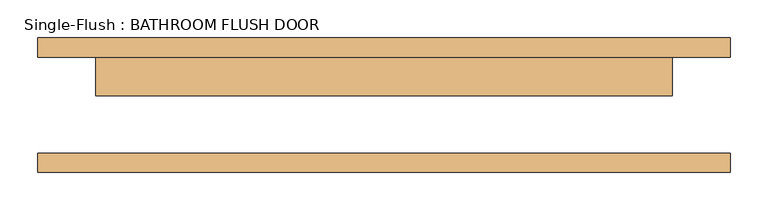
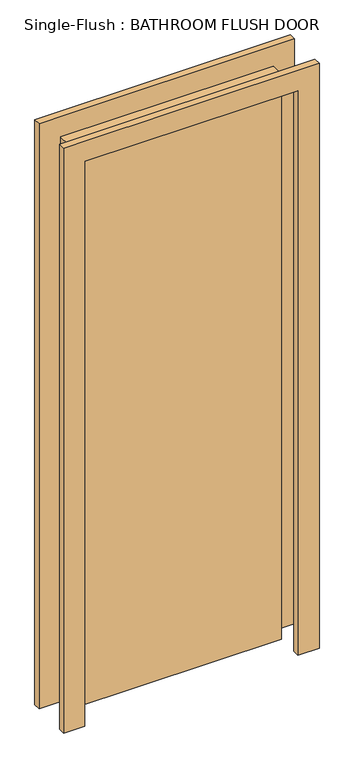
"""IFC4 building model written with IfcOpenShell, lengths in millimetres: door geometry, Single-Flush : BATHROOM FLUSH DOOR."""

from ifc_helpers import new_model, si_unit, frame, origin, origin_with_axes, place, context, project, spatial, polyline, outline, extrude, source, transform, mapped, element, save


def single_flush_bathroom_flush_door_4d6c7550(model_context):
    return source(origin(), model_context, "Body", "SweptSolid", [
        extrude(outline(polyline([(2209.8, -457.2), (0.0, -457.2), (0.0, -381.0), (2133.6, -381.0), (2133.6, 381.0), (0.0, 381.0), (0.0, 457.2), (2209.8, 457.2), (2209.8, -457.2)])), frame((0.0, 63.5, 0.0), z_axis=(0.0, 1.0, 0.0), x_axis=(0.0, 0.0, 1.0)), (0.0, 0.0, 1.0), 25.4),
        extrude(outline(polyline([(2209.8, 457.2), (2209.8, -457.2), (0.0, -457.2), (0.0, -381.0), (2133.6, -381.0), (2133.6, 381.0), (0.0, 381.0), (0.0, 457.2), (2209.8, 457.2)])), frame((0.0, -88.9, 0.0), z_axis=(0.0, 1.0, 0.0), x_axis=(0.0, 0.0, 1.0)), (0.0, 0.0, 1.0), 25.4),
        extrude(outline(polyline([(381.0, 12.7), (-381.0, 12.7), (-381.0, 63.5), (381.0, 63.5), (381.0, 12.7)])), origin_with_axes(), (0.0, 0.0, 1.0), 2133.6),
    ])


if __name__ == "__main__":
    model = new_model("IFC4")
    model_context = context("Model", 3, world=origin())
    ifc_project = project(units=[si_unit("LENGTHUNIT", "METRE", prefix="MILLI")], contexts=[model_context])
    site = spatial("IfcSite", under=ifc_project)
    building = spatial("IfcBuilding", under=site)
    placement = place(None, origin())
    single_flush_bathroom_flush_door_shape = single_flush_bathroom_flush_door_4d6c7550(model_context)
    element("IfcDoor", 1, ObjectType="Single-Flush : BATHROOM FLUSH DOOR", at=placement, inside=building, context=model_context, shape_type="MappedRepresentation", body=[
        mapped(single_flush_bathroom_flush_door_shape, transform((0.0, 0.0, 0.0), x_axis=(1.0, 0.0, 0.0), y_axis=(0.0, 1.0, 0.0), z_axis=(0.0, 0.0, 1.0))),
    ])
    save(model, "model.ifc")

# Revit data of these elements
# Type "Single-Flush : BATHROOM FLUSH DOOR"
#   Type Mark = "9"
#   Construction Type Id = "MDOOR"
#   Assembly Code = "C1020"
#   Analytic Construction = "Metal"
#   Thickness = 0' - 2"
#   Heat Transfer Coefficient (U) = 0.651978 BTU/(h·ft²·°F)
#   Height = 7' - 0"
#   Trim Projection Ext = 0' - 1"
#   Trim Projection Int = 0' - 1"
#   Trim Width = 0' - 3"
#   Width = 2' - 6"
#   Define Thermal Properties by = 1
#   Door Material = Door - Panel
#   Frame Material = Door - Frame
#   Visual Light Transmittance = 0
#   Solar Heat Gain Coefficient = 0
#   Function = (empty or 0)
#   Wall Closure = (empty or 0)
# Element 1 (IfcDoor, "Single-Flush : BATHROOM FLUSH DOOR")
#   Materials on its faces: "Door - Frame", "Door - Panel"
# Materials
#   "Door - Panel": class "Wood", colour RGB 210 159 95, transparency 0, Cost = 0
#   "Door - Frame": colour RGB 118 70 51, transparency 0, Cost = 0
